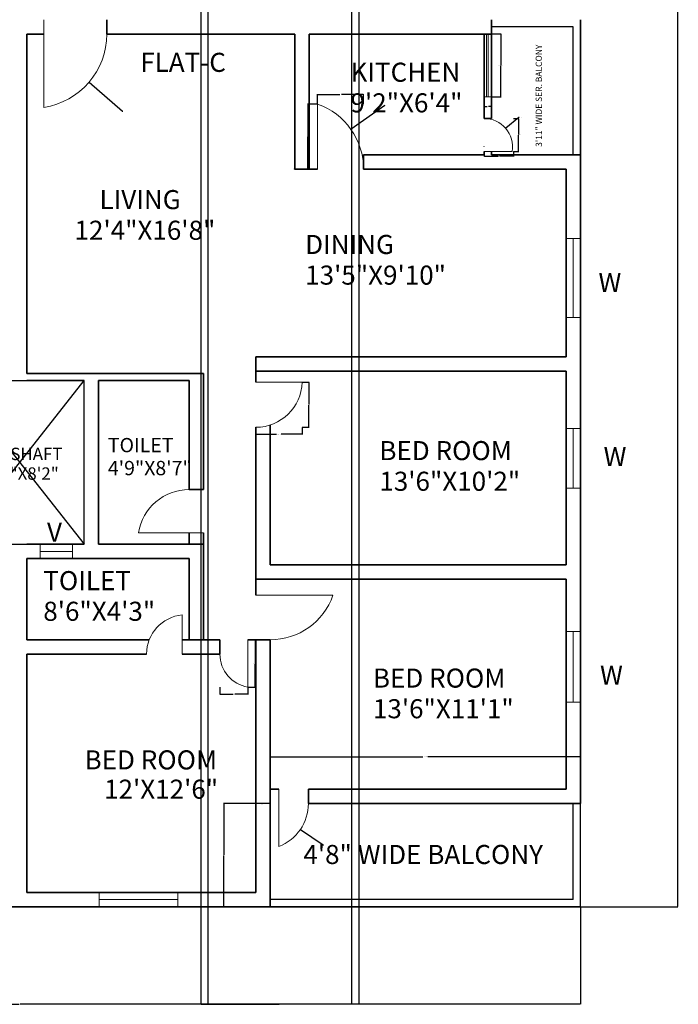
# Model space of a CAD drawing. Units: feet. Extents: x 5816 to 6644, y 25475 to 26788.
# Tile 2 of 23: x 6230 to 6644, y 25475 to 26094. Entities that reach past the tile are written whole.
import ezdxf

# ---------------------------------------------------------------- set-up
doc = ezdxf.new("R2010")
doc.units = ezdxf.units.FT
for name, color, linetype, lineweight in [('A-ANNO-DIMS', 2, 'Continuous', 13), ('A-ANNO-TEXT', 7, 'Continuous', 18), ('A-AREA-IDEN', 7, 'Continuous', 18), ('A-DOOR', 3, 'Continuous', 18), ('A-FLOR-RAIL', 8, 'Continuous', 25), ('A-FLOR-SHFT', 8, 'Continuous', 25), ('A-GLAZ', 4, 'Continuous', 18), ('A-WALL', 7, 'Continuous', 35)]:
    doc.layers.add(name, color=color, linetype=linetype, lineweight=lineweight)
doc.styles.get("Standard").update_dxf_attribs({"font": 'arial.ttf'})
doc.dimstyles.get("Standard").update_dxf_attribs({"dimtxt": 0.18, "dimasz": 0.18, "dimexe": 0.18, "dimexo": 0.0625, "dimgap": 0.09, "dimtad": 0, "dimtih": 1, "dimtoh": 1, "dimdec": 4, "dimzin": 0, "dimdsep": 46, "dimtxsty": 'Standard', "dimcen": 0.09, "dimadec": 0, "dimazin": 0, "dimtfac": 1, "dimtdec": 4, "dimtofl": 0, "dimtmove": 0, "dimatfit": 3, "dimfxl": 1, "dimtolj": 1, "dimtzin": 0, "dimarcsym": 0})

# ---------------------------------------------------------------- blocks, each defined once
blk = doc.blocks.new('DOOR-BALCONY')
blk.add_line((0, 36.11), (0, 0))
blk.add_arc((10.54, 9), 29.09, 111.24329, 180)
blk = doc.blocks.new('DOOR-BEDROOM-INNER')
blk.add_line((0, 29.82), (0, 0))
blk.add_arc((-3.45, 9), 21.11, 0, 80.59123)
blk = doc.blocks.new('DOOR-BEDROOM-BALCONY')
blk.add_line((-48.41, 0), (0, 0))
blk.add_arc((-9, -13.73), 41.74, 90, 160.78776)
blk = doc.blocks.new('DOOR-BEDROOM-SIDE')
blk.add_line((-28.98, 0), (0, 0))
blk.add_arc((0.03, -0.75), 29.02, 90, 178.52212)
blk = doc.blocks.new('DOOR-KITCHEN')
blk.add_line((0, -40.87), (0, 0))
blk.add_arc((14.45, 0), 43.35, 180, 250.52864)
blk = doc.blocks.new('DOOR-SERVICE-BALCONY')
blk.add_line((-17.56, 0), (0, 0))
blk.add_arc((0, -2.91), 17.8, 170.58679, 270)
blk = doc.blocks.new('DOOR-FLAT-ENTRY')
blk.add_line((0, 55.13), (0, 0))
blk.add_arc((7.05, 9.01), 46.66, 98.693, 180)
blk = doc.blocks.new('DOOR-BATH-ENSUITE')
blk.add_line((0, -24.59), (0, 0))
blk.add_arc((-2.33, 0.02), 24.72, 275.40734, 0)
blk = doc.blocks.new('DOOR-BATH-HALL')
blk.add_line((40.72, 0), (0, 0))
blk.add_arc((9, 4.86), 32.09, 270, 351.28818)
blk = doc.blocks.new('WIN-DINING')
for p, q in [((0, 0), (9, 0)), ((4.5, 0), (4.5, -49.84)), ((0, -49.84), (9, -49.84))]:
    blk.add_line(p, q)
blk = doc.blocks.new('WIN-BEDROOM-SIDE')
for p, q in [((0, 0), (9, 0)), ((4.5, 0), (4.5, -37.54)), ((0, -37.54), (9, -37.54))]:
    blk.add_line(p, q)
blk = doc.blocks.new('WIN-BEDROOM-BALCONY')
for p, q in [((0, 0), (9, 0)), ((4.5, 0), (4.5, -44.28)), ((0, -44.28), (9, -44.28))]:
    blk.add_line(p, q)
blk = doc.blocks.new('WIN-BEDROOM-INNER')
for p, q in [((49.5, 0), (49.5, -9)), ((0, 0), (0, -9)), ((0, -4.5), (49.5, -4.5))]:
    blk.add_line(p, q)
blk = doc.blocks.new('WIN-KITCHEN')
for p, q in [((0, 0), (4.5, 0)), ((2, 0), (2, -39.61)), ((3, 0), (3, -39.61))]:
    blk.add_line(p, q)
blk = doc.blocks.new('WIN-VENT-NARROW')
for p, q in [((0, 0), (0, -9)), ((20.24, 0), (20.24, -9)), ((0, -4.5), (20.24, -4.5))]:
    blk.add_line(p, q)
blk = doc.blocks.new('VENT-SHAFT')
for p, q in [((0, 0), (0, 103)), ((0, 103), (81, 103)), ((0, 103), (81, 0)), ((0, 0), (81, 103)), ((81, 103), (45, 103)), ((81, 0), (81, 103)), ((0, 0), (81, 0)), ((81, 0), (45, 0))]:
    blk.add_line(p, q)
blk = doc.blocks.new('RAIL-BALCONY-CORNER')
for p, q in [((0, 0), (0, -65)), ((0, 0), (195, 0)), ((4.5, -4.5), (4.5, -65)), ((4.5, -4.5), (195, -4.5))]:
    blk.add_line(p, q)
blk = doc.blocks.new('*D21')
at = {"layer": 'A-ANNO-DIMS', "color": 0, "lineweight": -2, "transparency": 16777216}
for p, q in [((6373.37, 25704.34), (6377.96, 25704.34)), ((6377.78, 25704.16), (6377.78, 25689.61)), ((6377.78, 25674.69), (6377.78, 25689.24)), ((6373.37, 25674.51), (6377.96, 25674.51))]:
    blk.add_line(p, q, dxfattribs=at)
at = {"layer": 'A-ANNO-DIMS', "color": 0, "transparency": 16777216}
for points in [[(6377.75, 25704.16), (6377.81, 25704.16), (6377.78, 25704.34)], [(6377.75, 25674.69), (6377.81, 25674.69), (6377.78, 25674.51)]]:
    blk.add_solid(points, dxfattribs=at)
at = {"layer": 'Defpoints', "color": 0, "transparency": 16777216}
for p in [(6373.31, 25704.34), (6373.31, 25674.51), (6377.78, 25674.51)]:
    blk.add_point(p, dxfattribs=at)
at = {"layer": 'A-ANNO-DIMS', "color": 0, "transparency": 16777216, "insert": (6377.78, 25689.42), "char_height": 0.18, "attachment_point": 5}
blk.add_mtext('\\A1;INNER BR DOOR 30 TYP.', dxfattribs=at)
blk = doc.blocks.new('*D22')
at = {"layer": 'A-ANNO-DIMS', "color": 0, "lineweight": -2, "transparency": 16777216}
for p, q in [((6355.65, 25674.45), (6355.65, 25669.86)), ((6373.31, 25674.45), (6373.31, 25669.86)), ((6355.83, 25670.04), (6363.96, 25670.04)), ((6373.13, 25670.04), (6365, 25670.04))]:
    blk.add_line(p, q, dxfattribs=at)
at = {"layer": 'A-ANNO-DIMS', "color": 0, "transparency": 16777216}
for points in [[(6355.83, 25670.07), (6355.83, 25670.01), (6355.65, 25670.04)], [(6373.13, 25670.07), (6373.13, 25670.01), (6373.31, 25670.04)]]:
    blk.add_solid(points, dxfattribs=at)
at = {"layer": 'Defpoints', "color": 0, "transparency": 16777216}
for p in [(6355.65, 25674.51), (6373.31, 25674.51), (6355.65, 25670.04)]:
    blk.add_point(p, dxfattribs=at)
at = {"layer": 'A-ANNO-DIMS', "color": 0, "transparency": 16777216, "insert": (6364.48, 25670.04), "char_height": 0.18, "attachment_point": 5}
blk.add_mtext('\\A1;18 TYP.', dxfattribs=at)
blk = doc.blocks.new('*D25')
at = {"layer": 'A-ANNO-DIMS', "color": 0, "lineweight": -2, "transparency": 16777216}
for p, q in [((6378.28, 25837.91), (6378.28, 25833.45)), ((6378.46, 25833.63), (6391.31, 25833.63)), ((6407.11, 25833.63), (6394.26, 25833.63)), ((6407.29, 25837.91), (6407.29, 25833.45))]:
    blk.add_line(p, q, dxfattribs=at)
at = {"layer": 'A-ANNO-DIMS', "color": 0, "transparency": 16777216}
for points in [[(6378.46, 25833.66), (6378.46, 25833.6), (6378.28, 25833.63)], [(6407.11, 25833.66), (6407.11, 25833.6), (6407.29, 25833.63)]]:
    blk.add_solid(points, dxfattribs=at)
at = {"layer": 'Defpoints', "color": 0, "transparency": 16777216}
for p in [(6378.28, 25837.98), (6378.28, 25833.63), (6407.29, 25837.98)]:
    blk.add_point(p, dxfattribs=at)
at = {"layer": 'A-ANNO-DIMS', "color": 0, "transparency": 16777216, "insert": (6392.78, 25833.63), "char_height": 0.18, "attachment_point": 5}
blk.add_mtext('\\A1;SIDE BR DOOR 29 TYP.', dxfattribs=at)
blk = doc.blocks.new('*D26')
at = {"layer": 'A-ANNO-DIMS', "color": 0, "lineweight": -2, "transparency": 16777216}
for p, q in [((6407.35, 25866.24), (6411.82, 25866.24)), ((6411.64, 25866.06), (6411.64, 25852.29)), ((6411.64, 25838.16), (6411.64, 25851.93)), ((6407.35, 25837.98), (6411.82, 25837.98))]:
    blk.add_line(p, q, dxfattribs=at)
at = {"layer": 'A-ANNO-DIMS', "color": 0, "transparency": 16777216}
for points in [[(6411.61, 25866.06), (6411.67, 25866.06), (6411.64, 25866.24)], [(6411.61, 25838.16), (6411.67, 25838.16), (6411.64, 25837.98)]]:
    blk.add_solid(points, dxfattribs=at)
at = {"layer": 'Defpoints', "color": 0, "transparency": 16777216}
for p in [(6407.29, 25866.24), (6407.29, 25837.98), (6411.64, 25837.98)]:
    blk.add_point(p, dxfattribs=at)
at = {"layer": 'A-ANNO-DIMS', "color": 0, "transparency": 16777216, "insert": (6411.64, 25852.11), "char_height": 0.18, "attachment_point": 5}
blk.add_mtext('\\A1;28 TYP.', dxfattribs=at)
blk = doc.blocks.new('*D27')
at = {"layer": 'A-ANNO-DIMS', "color": 0, "lineweight": -2, "transparency": 16777216}
for p, q in [((6417.03, 26041.21), (6410.78, 26041.21)), ((6410.96, 26041.03), (6410.96, 26020.95)), ((6410.96, 26000.52), (6410.96, 26020.59)), ((6417.03, 26000.34), (6410.78, 26000.34))]:
    blk.add_line(p, q, dxfattribs=at)
at = {"layer": 'A-ANNO-DIMS', "color": 0, "transparency": 16777216}
for points in [[(6410.93, 26041.03), (6410.99, 26041.03), (6410.96, 26041.21)], [(6410.93, 26000.52), (6410.99, 26000.52), (6410.96, 26000.34)]]:
    blk.add_solid(points, dxfattribs=at)
at = {"layer": 'Defpoints', "color": 0, "transparency": 16777216}
for p in [(6417.09, 26041.21), (6410.96, 26000.34), (6417.09, 26000.34)]:
    blk.add_point(p, dxfattribs=at)
at = {"layer": 'A-ANNO-DIMS', "color": 0, "transparency": 16777216, "insert": (6410.96, 26020.77), "char_height": 0.18, "attachment_point": 5}
blk.add_mtext('\\A1;KITCHEN DOOR 41 TYP.', dxfattribs=at)
blk = doc.blocks.new('*D28')
at = {"layer": 'A-ANNO-DIMS', "color": 0, "lineweight": -2, "transparency": 16777216}
for p, q in [((6417.09, 26041.27), (6417.09, 26047.52)), ((6417.27, 26047.34), (6431.01, 26047.34)), ((6445.81, 26047.34), (6432.07, 26047.34)), ((6445.99, 26041.27), (6445.99, 26047.52))]:
    blk.add_line(p, q, dxfattribs=at)
at = {"layer": 'A-ANNO-DIMS', "color": 0, "transparency": 16777216}
for points in [[(6417.27, 26047.37), (6417.27, 26047.31), (6417.09, 26047.34)], [(6445.81, 26047.37), (6445.81, 26047.31), (6445.99, 26047.34)]]:
    blk.add_solid(points, dxfattribs=at)
at = {"layer": 'Defpoints', "color": 0, "transparency": 16777216}
for p in [(6417.09, 26047.34), (6417.09, 26041.21), (6445.99, 26041.21)]:
    blk.add_point(p, dxfattribs=at)
at = {"layer": 'A-ANNO-DIMS', "color": 0, "transparency": 16777216, "insert": (6431.54, 26047.34), "char_height": 0.18, "attachment_point": 5}
blk.add_mtext('\\A1;29 TYP.', dxfattribs=at)
blk = doc.blocks.new('*D29')
at = {"layer": 'A-ANNO-DIMS', "color": 0, "lineweight": -2, "transparency": 16777216}
for p, q in [((6540.29, 26032.22), (6543.51, 26032.22)), ((6543.33, 26032.04), (6543.33, 26022.05)), ((6543.33, 26011.7), (6543.33, 26021.69)), ((6540.29, 26011.52), (6543.51, 26011.52))]:
    blk.add_line(p, q, dxfattribs=at)
at = {"layer": 'A-ANNO-DIMS', "color": 0, "transparency": 16777216}
for points in [[(6543.3, 26032.04), (6543.36, 26032.04), (6543.33, 26032.22)], [(6543.3, 26011.7), (6543.36, 26011.7), (6543.33, 26011.52)]]:
    blk.add_solid(points, dxfattribs=at)
at = {"layer": 'Defpoints', "color": 0, "transparency": 16777216}
for p in [(6540.23, 26032.22), (6540.23, 26011.52), (6543.33, 26011.52)]:
    blk.add_point(p, dxfattribs=at)
at = {"layer": 'A-ANNO-DIMS', "color": 0, "transparency": 16777216, "insert": (6543.33, 26021.87), "char_height": 0.18, "attachment_point": 5}
blk.add_mtext('\\A1;SERVICE DOOR 21 TYP.', dxfattribs=at)
blk = doc.blocks.new('*D30')
at = {"layer": 'A-ANNO-DIMS', "color": 0, "lineweight": -2, "transparency": 16777216}
for p, q in [((6521.81, 26011.45), (6521.81, 26008.23)), ((6521.99, 26008.41), (6530.5, 26008.41)), ((6540.05, 26008.41), (6531.54, 26008.41)), ((6540.23, 26011.45), (6540.23, 26008.23))]:
    blk.add_line(p, q, dxfattribs=at)
at = {"layer": 'A-ANNO-DIMS', "color": 0, "transparency": 16777216}
for points in [[(6521.99, 26008.44), (6521.99, 26008.38), (6521.81, 26008.41)], [(6540.05, 26008.44), (6540.05, 26008.38), (6540.23, 26008.41)]]:
    blk.add_solid(points, dxfattribs=at)
at = {"layer": 'Defpoints', "color": 0, "transparency": 16777216}
for p in [(6521.81, 26011.52), (6521.81, 26008.41), (6540.23, 26011.52)]:
    blk.add_point(p, dxfattribs=at)
at = {"layer": 'A-ANNO-DIMS', "color": 0, "transparency": 16777216, "insert": (6531.02, 26008.41), "char_height": 0.18, "attachment_point": 5}
blk.add_mtext('\\A1;18 TYP.', dxfattribs=at)
blk = doc.blocks.new('*D45')
at = {"layer": 'A-ANNO-DIMS', "color": 0, "lineweight": -2, "transparency": 16777216}
for p, q in [((6526.37, 26085.34), (6532.43, 26085.34)), ((6532.25, 26085.16), (6532.25, 26065.72)), ((6532.25, 26045.91), (6532.25, 26065.35)), ((6526.37, 26045.73), (6532.43, 26045.73))]:
    blk.add_line(p, q, dxfattribs=at)
at = {"layer": 'A-ANNO-DIMS', "color": 0, "transparency": 16777216}
for points in [[(6532.22, 26085.16), (6532.28, 26085.16), (6532.25, 26085.34)], [(6532.22, 26045.91), (6532.28, 26045.91), (6532.25, 26045.73)]]:
    blk.add_solid(points, dxfattribs=at)
at = {"layer": 'Defpoints', "color": 0, "transparency": 16777216}
for p in [(6526.31, 26085.34), (6526.31, 26045.73), (6532.25, 26045.73)]:
    blk.add_point(p, dxfattribs=at)
at = {"layer": 'A-ANNO-DIMS', "color": 0, "transparency": 16777216, "insert": (6532.25, 26065.53), "char_height": 0.18, "attachment_point": 5}
blk.add_mtext('\\A1;KITCHEN WINDOW 40 TYP.', dxfattribs=at)
blk = doc.blocks.new('*D46')
at = {"layer": 'A-ANNO-DIMS', "color": 0, "lineweight": -2, "transparency": 16777216}
for p, q in [((6521.81, 26045.67), (6521.81, 26039.61)), ((6526.31, 26045.67), (6526.31, 26039.61)), ((6521.99, 26039.79), (6523.6, 26039.79)), ((6526.13, 26039.79), (6524.52, 26039.79))]:
    blk.add_line(p, q, dxfattribs=at)
at = {"layer": 'A-ANNO-DIMS', "color": 0, "transparency": 16777216}
for points in [[(6521.99, 26039.82), (6521.99, 26039.76), (6521.81, 26039.79)], [(6526.13, 26039.82), (6526.13, 26039.76), (6526.31, 26039.79)]]:
    blk.add_solid(points, dxfattribs=at)
at = {"layer": 'Defpoints', "color": 0, "transparency": 16777216}
for p in [(6521.81, 26045.73), (6526.31, 26045.73), (6521.81, 26039.79)]:
    blk.add_point(p, dxfattribs=at)
at = {"layer": 'A-ANNO-DIMS', "color": 0, "transparency": 16777216, "insert": (6524.06, 26039.79), "char_height": 0.18, "attachment_point": 5}
blk.add_mtext('\\A1;5 TYP.', dxfattribs=at)
blk = doc.blocks.new('*D47')
at = {"layer": 'A-ANNO-DIMS', "color": 0, "lineweight": -2, "transparency": 16777216}
for p, q in [((6387.31, 25601.4), (6387.31, 25630.77)), ((6387.49, 25630.59), (6483.27, 25630.59)), ((6582.13, 25630.59), (6486.36, 25630.59)), ((6582.31, 25601.4), (6582.31, 25630.77))]:
    blk.add_line(p, q, dxfattribs=at)
at = {"layer": 'A-ANNO-DIMS', "color": 0, "transparency": 16777216}
for points in [[(6387.49, 25630.62), (6387.49, 25630.56), (6387.31, 25630.59)], [(6582.13, 25630.62), (6582.13, 25630.56), (6582.31, 25630.59)]]:
    blk.add_solid(points, dxfattribs=at)
at = {"layer": 'Defpoints', "color": 0, "transparency": 16777216}
for p in [(6387.31, 25630.59), (6387.31, 25601.34), (6582.31, 25601.34)]:
    blk.add_point(p, dxfattribs=at)
at = {"layer": 'A-ANNO-DIMS', "color": 0, "transparency": 16777216, "insert": (6484.81, 25630.59), "char_height": 0.18, "attachment_point": 5}
blk.add_mtext('\\A1;BALCONY RAIL 195 TYP.', dxfattribs=at)
blk = doc.blocks.new('*D48')
at = {"layer": 'A-ANNO-DIMS', "color": 0, "lineweight": -2, "transparency": 16777216}
for p, q in [((6387.25, 25601.34), (6357.88, 25601.34)), ((6358.06, 25601.16), (6358.06, 25569.02)), ((6358.06, 25536.52), (6358.06, 25568.65)), ((6387.25, 25536.34), (6357.88, 25536.34))]:
    blk.add_line(p, q, dxfattribs=at)
at = {"layer": 'A-ANNO-DIMS', "color": 0, "transparency": 16777216}
for points in [[(6358.03, 25601.16), (6358.09, 25601.16), (6358.06, 25601.34)], [(6358.03, 25536.52), (6358.09, 25536.52), (6358.06, 25536.34)]]:
    blk.add_solid(points, dxfattribs=at)
at = {"layer": 'Defpoints', "color": 0, "transparency": 16777216}
for p in [(6387.31, 25601.34), (6358.06, 25536.34), (6387.31, 25536.34)]:
    blk.add_point(p, dxfattribs=at)
at = {"layer": 'A-ANNO-DIMS', "color": 0, "transparency": 16777216, "insert": (6358.06, 25568.84), "char_height": 0.18, "attachment_point": 5}
blk.add_mtext('\\A1;65 TYP.', dxfattribs=at)
blk = doc.blocks.new('*D55')
at = {"layer": 'A-ANNO-DIMS', "color": 0, "lineweight": -2, "transparency": 16777216}
for p, q in [((5877.31, 25536.27), (5877.31, 25475.01)), ((6582.31, 25536.27), (6582.31, 25475.01)), ((5877.49, 25475.19), (6229.52, 25475.19)), ((6582.13, 25475.19), (6230.1, 25475.19))]:
    blk.add_line(p, q, dxfattribs=at)
at = {"layer": 'A-ANNO-DIMS', "color": 0, "transparency": 16777216}
for points in [[(5877.49, 25475.22), (5877.49, 25475.16), (5877.31, 25475.19)], [(6582.13, 25475.22), (6582.13, 25475.16), (6582.31, 25475.19)]]:
    blk.add_solid(points, dxfattribs=at)
at = {"layer": 'Defpoints', "color": 0, "transparency": 16777216}
for p in [(5877.31, 25536.34), (6582.31, 25536.34), (6582.31, 25475.19)]:
    blk.add_point(p, dxfattribs=at)
at = {"layer": 'A-ANNO-DIMS', "color": 0, "transparency": 16777216, "insert": (6229.81, 25475.19), "char_height": 0.18, "attachment_point": 5}
blk.add_mtext('\\A1;705', dxfattribs=at)
blk = doc.blocks.new('*D56')
at = {"layer": 'A-ANNO-DIMS', "color": 0, "lineweight": -2, "transparency": 16777216}
for p, q in [((6582.37, 26726.58), (6643.64, 26726.58)), ((6643.46, 26726.4), (6643.46, 26131.64)), ((6643.46, 25536.52), (6643.46, 26131.28)), ((6582.37, 25536.34), (6643.64, 25536.34))]:
    blk.add_line(p, q, dxfattribs=at)
at = {"layer": 'A-ANNO-DIMS', "color": 0, "transparency": 16777216}
for points in [[(6643.43, 26726.4), (6643.49, 26726.4), (6643.46, 26726.58)], [(6643.43, 25536.52), (6643.49, 25536.52), (6643.46, 25536.34)]]:
    blk.add_solid(points, dxfattribs=at)
at = {"layer": 'Defpoints', "color": 0, "transparency": 16777216}
for p in [(6582.31, 26726.58), (6643.46, 26726.58), (6582.31, 25536.34)]:
    blk.add_point(p, dxfattribs=at)
at = {"layer": 'A-ANNO-DIMS', "color": 0, "transparency": 16777216, "insert": (6643.46, 26131.46), "char_height": 0.18, "attachment_point": 5}
blk.add_mtext('\\A1;1190.2', dxfattribs=at)
blk = doc.blocks.new('*D59')
at = {"layer": 'A-ANNO-DIMS', "color": 0, "lineweight": -2, "transparency": 16777216}
for p, q in [((6343.68, 26168.52), (6343.68, 25475.01)), ((6442.98, 26168.59), (6442.98, 25475.01)), ((6343.86, 25475.19), (6393, 25475.19)), ((6442.8, 25475.19), (6393.65, 25475.19))]:
    blk.add_line(p, q, dxfattribs=at)
at = {"layer": 'A-ANNO-DIMS', "color": 0, "transparency": 16777216}
for points in [[(6343.86, 25475.22), (6343.86, 25475.16), (6343.68, 25475.19)], [(6442.8, 25475.22), (6442.8, 25475.16), (6442.98, 25475.19)]]:
    blk.add_solid(points, dxfattribs=at)
at = {"layer": 'Defpoints', "color": 0, "transparency": 16777216}
for p in [(6343.68, 26168.58), (6442.98, 26168.65), (6442.98, 25475.19)]:
    blk.add_point(p, dxfattribs=at)
at = {"layer": 'A-ANNO-DIMS', "color": 0, "transparency": 16777216, "insert": (6393.33, 25475.19), "char_height": 0.18, "attachment_point": 5}
blk.add_mtext('\\A1;99.3', dxfattribs=at)
blk = doc.blocks.new('*D73')
at = {"layer": 'A-ANNO-DIMS', "color": 0, "lineweight": -2, "transparency": 16777216}
for p, q in [((6348.18, 26111.07), (6348.18, 25475.01)), ((6438.48, 26111.07), (6438.48, 25475.01)), ((6348.36, 25475.19), (6393, 25475.19)), ((6438.3, 25475.19), (6393.65, 25475.19))]:
    blk.add_line(p, q, dxfattribs=at)
at = {"layer": 'A-ANNO-DIMS', "color": 0, "transparency": 16777216}
for points in [[(6348.36, 25475.22), (6348.36, 25475.16), (6348.18, 25475.19)], [(6438.3, 25475.22), (6438.3, 25475.16), (6438.48, 25475.19)]]:
    blk.add_solid(points, dxfattribs=at)
at = {"layer": 'Defpoints', "color": 0, "transparency": 16777216}
for p in [(6348.18, 26111.13), (6438.48, 26111.13), (6438.48, 25475.19)]:
    blk.add_point(p, dxfattribs=at)
at = {"layer": 'A-ANNO-DIMS', "color": 0, "transparency": 16777216, "insert": (6393.33, 25475.19), "char_height": 0.18, "attachment_point": 5}
blk.add_mtext('\\A1;90.3', dxfattribs=at)
blk = doc.blocks.new('*D74')
at = {"layer": 'A-ANNO-DIMS', "color": 0, "lineweight": -2, "transparency": 16777216}
for p, q in [((6237.79, 26085.33), (6237.97, 26085.33)), ((6237.88, 26085.24), (6237.88, 26085.42)), ((6294.52, 26036.69), (6273.42, 26054.81)), ((6294.7, 26036.69), (6294.52, 26036.69))]:
    blk.add_line(p, q, dxfattribs=at)
at = {"layer": 'A-ANNO-DIMS', "color": 0, "transparency": 16777216}
blk.add_solid([(6273.44, 26054.84), (6273.4, 26054.79), (6273.28, 26054.93)], dxfattribs=at)
at = {"layer": 'Defpoints', "color": 0, "transparency": 16777216}
for p in [(6237.88, 26085.33), (6273.28, 26054.93)]:
    blk.add_point(p, dxfattribs=at)
at = {"layer": 'A-ANNO-DIMS', "color": 0, "transparency": 16777216, "insert": (6295.38, 26036.69), "char_height": 0.18, "attachment_point": 5}
blk.add_mtext('\\A1;4X R46.66', dxfattribs=at)
blk = doc.blocks.new('*D75')
at = {"layer": 'A-ANNO-DIMS', "color": 0, "lineweight": -2, "transparency": 16777216}
for p, q in [((6459.27, 26040.38), (6438.18, 26025.47)), ((6459.45, 26040.38), (6459.27, 26040.38)), ((6402.55, 26000.34), (6402.73, 26000.34)), ((6402.64, 26000.25), (6402.64, 26000.43))]:
    blk.add_line(p, q, dxfattribs=at)
at = {"layer": 'A-ANNO-DIMS', "color": 0, "transparency": 16777216}
blk.add_solid([(6438.17, 26025.49), (6438.2, 26025.44), (6438.04, 26025.36)], dxfattribs=at)
at = {"layer": 'Defpoints', "color": 0, "transparency": 16777216}
for p in [(6438.04, 26025.36), (6402.64, 26000.34)]:
    blk.add_point(p, dxfattribs=at)
at = {"layer": 'A-ANNO-DIMS', "color": 0, "transparency": 16777216, "insert": (6460.13, 26040.38), "char_height": 0.18, "attachment_point": 5}
blk.add_mtext('\\A1;4X R43.35', dxfattribs=at)
blk = doc.blocks.new('*D78')
at = {"layer": 'A-ANNO-DIMS', "color": 0, "lineweight": -2, "transparency": 16777216}
for p, q in [((6382.13, 25601.34), (6382.31, 25601.34)), ((6382.22, 25601.25), (6382.22, 25601.43)), ((6420.64, 25575.06), (6406.38, 25584.81)), ((6420.82, 25575.06), (6420.64, 25575.06))]:
    blk.add_line(p, q, dxfattribs=at)
at = {"layer": 'A-ANNO-DIMS', "color": 0, "transparency": 16777216}
blk.add_solid([(6406.4, 25584.83), (6406.36, 25584.78), (6406.23, 25584.91)], dxfattribs=at)
at = {"layer": 'Defpoints', "color": 0, "transparency": 16777216}
for p in [(6382.22, 25601.34), (6406.23, 25584.91)]:
    blk.add_point(p, dxfattribs=at)
at = {"layer": 'A-ANNO-DIMS', "color": 0, "transparency": 16777216, "insert": (6421.49, 25575.06), "char_height": 0.18, "attachment_point": 5}
blk.add_mtext('\\A1;4X R29.09', dxfattribs=at)
blk = doc.blocks.new('*D82')
at = {"layer": 'A-ANNO-DIMS', "color": 0, "lineweight": -2, "transparency": 16777216}
for p, q in [((6543.53, 26032.84), (6535.52, 26026.05)), ((6543.71, 26032.84), (6543.53, 26032.84)), ((6521.72, 26014.43), (6521.9, 26014.43)), ((6521.81, 26014.34), (6521.81, 26014.52))]:
    blk.add_line(p, q, dxfattribs=at)
at = {"layer": 'A-ANNO-DIMS', "color": 0, "transparency": 16777216}
blk.add_solid([(6535.5, 26026.08), (6535.54, 26026.03), (6535.39, 26025.94)], dxfattribs=at)
at = {"layer": 'Defpoints', "color": 0, "transparency": 16777216}
for p in [(6535.39, 26025.94), (6521.81, 26014.43)]:
    blk.add_point(p, dxfattribs=at)
at = {"layer": 'A-ANNO-DIMS', "color": 0, "transparency": 16777216, "insert": (6544.46, 26032.84), "char_height": 0.18, "attachment_point": 5}
blk.add_mtext('\\A1;4X R17.798', dxfattribs=at)

msp = doc.modelspace()

# ---------------------------------------------------------------- linework, layer by layer
at = {"layer": 'A-FLOR-RAIL'}
msp.add_lwpolyline([(6577.8119, 26009.3368), (6577.8119, 26089.8368), (6526.3119, 26089.8368)], dxfattribs=at)
at = {"layer": 'A-WALL'}
for p, q in [((6284.5408, 26085.3298), (6284.5408, 26094.3368)), ((6526.3119, 26032.2246), (6526.3119, 26094.3368)), ((6582.3119, 26000.3368), (6582.3119, 26094.3368)), ((6244.9332, 26085.3368), (6234.3119, 26085.3368)), ((6234.3119, 25871.8368), (6234.3119, 26085.3368)), ((6402.8119, 26085.3368), (6284.5408, 26085.3368)), ((6402.8119, 26085.3368), (6402.8119, 26009.3368)), ((6526.3119, 26085.3368), (6411.8119, 26085.3368)), ((6411.8119, 26085.3368), (6411.8119, 26000.3368)), ((6521.8119, 26032.2246), (6521.8119, 26085.3368)), ((6526.3119, 26032.2246), (6521.8119, 26032.2246)), ((6402.8119, 26009.3368), (6402.8119, 26000.3368)), ((6521.8119, 26009.3368), (6445.9911, 26009.3368)), ((6445.9911, 26000.3368), (6445.9911, 26009.3368)), ((6521.8119, 26009.3368), (6521.8119, 26011.5155)), ((6526.3119, 26009.3368), (6526.3119, 26011.5155)), ((6573.3119, 26009.3368), (6526.3119, 26009.3368)), ((6573.3119, 26009.3368), (6582.3119, 26009.3368)), ((6582.3119, 25610.3368), (6582.3119, 26009.3368)), ((6582.3119, 25751.3368), (6582.3119, 26009.3368)), ((6417.0917, 26000.3368), (6402.8119, 26000.3368)), ((6573.3119, 26000.3368), (6445.9911, 26000.3368)), ((6573.3119, 25882.3368), (6573.3119, 26000.3368)), ((6582.3119, 25882.3368), (6582.3119, 26000.3368)), ((6573.3119, 25882.3368), (6378.3119, 25882.3368)), ((6378.3119, 25866.2444), (6378.3119, 25882.3368)), ((6336.3119, 25871.8368), (6234.3119, 25871.8368)), ((6336.3119, 25871.8368), (6345.3119, 25871.8368)), ((6345.3119, 25798.8236), (6345.3119, 25871.8368)), ((6573.3119, 25873.3368), (6378.3119, 25873.3368)), ((6573.3119, 25751.3368), (6573.3119, 25873.3368)), ((6336.3119, 25867.3368), (6279.3119, 25867.3368)), ((6279.3119, 25867.3368), (6279.3119, 25764.3368)), ((6336.3119, 25798.8236), (6336.3119, 25867.3368)), ((6387.3119, 25751.3368), (6387.3119, 25839.4181)), ((6378.3119, 25732.3387), (6378.3119, 25837.9771)), ((6336.3119, 25798.8236), (6345.3119, 25798.8236)), ((6336.3119, 25764.3368), (6336.3119, 25771.5927)), ((6345.3119, 25704.3368), (6345.3119, 25771.5927)), ((6345.3119, 25764.3368), (6279.3119, 25764.3368)), ((6336.3119, 25755.3368), (6234.3119, 25755.3368)), ((6234.3119, 25755.3368), (6234.3119, 25704.3368)), ((6336.3119, 25704.3368), (6336.3119, 25755.3368)), ((6573.3119, 25751.3368), (6387.3119, 25751.3368)), ((6573.3119, 25742.3368), (6378.3119, 25742.3368)), ((6378.3119, 25742.3368), (6378.3119, 25732.3387)), ((6573.3119, 25610.3368), (6573.3119, 25742.3368)), ((6234.3119, 25704.3368), (6311.248, 25704.3368)), ((6234.3119, 25704.3368), (6311.248, 25704.3368)), ((6331.936, 25704.3368), (6355.6538, 25704.3368)), ((6331.936, 25704.3368), (6336.3119, 25704.3368)), ((6355.6538, 25695.3368), (6355.6538, 25704.3368)), ((6373.3112, 25704.3368), (6387.3119, 25704.3368)), ((6378.3119, 25704.3368), (6378.3119, 25594.1569)), ((6387.3119, 25704.3368), (6387.3119, 25594.1569)), ((6234.3119, 25545.3368), (6234.3119, 25695.3368)), ((6234.3119, 25695.3368), (6309.5426, 25695.3368)), ((6331.936, 25695.3368), (6355.6538, 25695.3368)), ((6392.7622, 25610.3368), (6387.3119, 25610.3368)), ((6573.3119, 25610.3368), (6411.3119, 25610.3368)), ((6411.3119, 25610.3368), (6411.3119, 25601.3368)), ((6582.3119, 25601.3368), (6582.3119, 25610.3368)), ((6378.3119, 25601.3368), (6378.3119, 25545.3368)), ((6387.3119, 25601.3368), (6387.3119, 25536.3368)), ((6582.3119, 25601.3368), (6411.3119, 25601.3368)), ((6378.3119, 25545.3368), (6234.3119, 25545.3368)), ((5877.3119, 25536.3368), (6279.7398, 25536.3368)), ((6582.3119, 25536.3368), (6234.3119, 25536.3368))]:
    msp.add_line(p, q, dxfattribs=at)

# ---------------------------------------------------------------- block references
at = {"layer": 'A-DOOR', "rotation": 180}
for name, p in [('DOOR-FLAT-ENTRY', (6244.9332, 26094.3368)), ('DOOR-KITCHEN', (6417.0917, 26000.3368)), ('DOOR-SERVICE-BALCONY', (6521.8119, 26011.5155)), ('DOOR-BEDROOM-SIDE', (6378.3119, 25866.2444)), ('DOOR-BATH-HALL', (6345.3119, 25771.5927)), ('DOOR-BEDROOM-BALCONY', (6378.3119, 25732.3387)), ('DOOR-BATH-ENSUITE', (6331.936, 25695.3368)), ('DOOR-BEDROOM-INNER', (6373.3112, 25704.3368)), ('DOOR-BALCONY', (6392.7622, 25610.3368))]:
    msp.add_blockref(name, p, dxfattribs=at)
at = {"layer": 'A-FLOR-RAIL', "rotation": 180}
msp.add_blockref('RAIL-BALCONY-CORNER', (6582.3119, 25536.3368), dxfattribs=at)
at = {"layer": 'A-FLOR-SHFT'}
msp.add_blockref('VENT-SHAFT', (6189.3119, 25764.3368), dxfattribs=at)
at = {"layer": 'A-GLAZ', "rotation": 180}
for name, p in [('WIN-KITCHEN', (6526.3119, 26045.731)), ('WIN-DINING', (6582.3119, 25906.9414)), ('WIN-BEDROOM-BALCONY', (6582.3119, 25665.1277))]:
    msp.add_blockref(name, p, dxfattribs=at)
at = {"layer": 'A-GLAZ'}
for name, p in [('WIN-BEDROOM-SIDE', (6573.3119, 25837.1796)), ('WIN-VENT-NARROW', (6242.7596, 25764.3368)), ('WIN-BEDROOM-INNER', (6279.7398, 25545.3368))]:
    msp.add_blockref(name, p, dxfattribs=at)

# ---------------------------------------------------------------- texts
at = {"layer": 'A-ANNO-DIMS'}
for s, height, p in [('9\'2"X6\'4"', 12, (6437.7909, 26036.0213)), ('12\'4"X16\'8"', 12, (6264.2851, 25955.8889)), ('13\'5"X9\'10"', 12, (6409.2785, 25927.6758)), ('4\'9"X8\'7"', 8.98988, (6285.2405, 25807.8127)), ('6\'7"X8\'2"', 7.77416, (6208.7805, 25804.961)), ('13\'6"X10\'2"', 12, (6455.9147, 25798.0042)), ('8\'6"X4\'3"', 12, (6244.6415, 25716.2184)), ('13\'6"X11\'1"', 12, (6451.861, 25654.9247)), ('12\'X12\'6"', 12, (6282.8763, 25604.3235))]:
    msp.add_text(s, height=height, dxfattribs=at).set_placement(p)
at = {"layer": 'A-ANNO-TEXT'}
for s, p in [('W', (6593.636, 25923.074)), ('W', (6596.8674, 25813.5301)), ('V', (6246.9756, 25766.0074)), ('W', (6594.6249, 25676.0997))]:
    msp.add_text(s, height=12, dxfattribs=at).set_placement(p)
at = {"layer": 'A-AREA-IDEN'}
msp.add_text('3\'11" WIDE SER. BALCONY', height=3.901456, rotation=90, dxfattribs=at).set_placement((6558.0829, 26014.3721))
for s, height, p in [('FLAT-C', 12, (6305.6106, 26061.5111)), ('KITCHEN', 12, (6437.7909, 26055.2983)), ('LIVING', 12, (6279.9748, 25975.1658)), ('DINING', 12, (6409.2785, 25946.9527)), ('TOILET', 8.98988, (6285.2405, 25822.2542)), ('BED ROOM', 12, (6455.9147, 25817.2811)), ('VENT SHAFT', 7.77416, (6195.225, 25817.342)), ('TOILET', 12, (6244.6415, 25735.4953)), ('BED ROOM', 12, (6451.861, 25674.2016)), ('BED ROOM', 12, (6270.5851, 25622.7534)), ('4\'8" WIDE BALCONY', 12, (6408.1538, 25563.2479))]:
    msp.add_text(s, height=height, dxfattribs=at).set_placement(p)

# ---------------------------------------------------------------- dimensions: what is measured, and where the dimension line sits
at = {"layer": 'A-ANNO-DIMS'}
dim = msp.add_linear_dim(base=(6643.4619, 26726.5846), p1=(6582.3119, 25536.3368), p2=(6582.3119, 26726.5846), angle=90, dimstyle='Standard', override={"dimdec": 1, "dimlfac": 1, "dimrnd": 0, "dimzin": 0, "dimdsep": 46, "dimlunit": 2}, dxfattribs=at)
dim.commit()
dim.dimension.update_dxf_attribs({"geometry": '*D56', "text_midpoint": (6643.4619, 26131.4607)})
for base, p1, p2, override, picture, middle in [((6442.9781, 25475.1868), (6343.6763, 26168.5846), (6442.9781, 26168.6509), {"dimdec": 1, "dimlfac": 1, "dimrnd": 0, "dimzin": 0, "dimdsep": 46, "dimlunit": 2}, '*D59', (6393.3272, 25475.1868)), ((6438.4781, 25475.1868), (6348.1763, 26111.129), (6438.4781, 26111.129), {"dimdec": 1, "dimlfac": 1, "dimrnd": 0, "dimzin": 0, "dimdsep": 46, "dimlunit": 2}, '*D73', (6393.3272, 25475.1868)), ((6582.3119, 25475.1868), (5877.3119, 25536.3368), (6582.3119, 25536.3368), {"dimdec": 0, "dimlfac": 1, "dimrnd": 0, "dimzin": 0, "dimdsep": 46, "dimlunit": 2}, '*D55', (6229.8119, 25475.1868))]:
    dim = msp.add_linear_dim(base=base, p1=p1, p2=p2, dimstyle='Standard', override=override, dxfattribs=at)
    dim.commit()
    dim.dimension.update_dxf_attribs({"geometry": picture, "text_midpoint": middle})
for center, mpoint, override, picture, middle in [((6237.881, 26085.3298), (6273.2802, 26054.9319), {"dimdec": 2, "dimlfac": 1, "dimrnd": 0, "dimzin": 0, "dimdsep": 46, "dimlunit": 2}, '*D74', (6295.3765, 26036.6931)), ((6402.6419, 26000.3368), (6438.0364, 26025.3643), {"dimdec": 2, "dimlfac": 1, "dimrnd": 0, "dimzin": 0, "dimdsep": 46, "dimlunit": 2}, '*D75', (6460.1307, 26040.3808)), ((6521.8119, 26014.4264), (6535.3869, 26025.937), {"dimdec": 3, "dimlfac": 1, "dimrnd": 0, "dimzin": 0, "dimdsep": 46, "dimlunit": 2}, '*D82', (6544.459, 26032.8433)), ((6382.2221, 25601.3368), (6406.2307, 25584.9112), {"dimdec": 2, "dimlfac": 1, "dimrnd": 0, "dimzin": 0, "dimdsep": 46, "dimlunit": 2}, '*D78', (6421.4929, 25575.0558))]:
    dim = msp.add_radius_dim(center=center, mpoint=mpoint, text='4X <>', dimstyle='Standard', override=override, dxfattribs=at)
    dim.commit()
    dim.dimension.update_dxf_attribs({"geometry": picture, "text_midpoint": middle, "dimtype": 164})
for base, p1, p2, angle, text, picture, middle in [((6532.2527, 26045.731), (6526.3119, 26085.3368), (6526.3119, 26045.731), 270, 'KITCHEN WINDOW <> TYP.', '*D45', (6532.2527, 26065.5339)), ((6417.0917, 26047.3373), (6445.9911, 26041.2068), (6417.0917, 26041.2068), 180, '<> TYP.', '*D28', (6431.5414, 26047.3373)), ((6521.8118536836, 26039.7901388672), (6526.3118536836, 26045.7310044178), (6521.8118536836, 26045.7310044178), 180, '<> TYP.', '*D46', (6524.0618536836, 26039.7901388672)), ((6410.9612, 26000.3368), (6417.0917, 26041.2068), (6417.0917, 26000.3368), 270, 'KITCHEN DOOR <> TYP.', '*D27', (6410.9612, 26020.7718)), ((6543.332, 26011.5155), (6540.2256, 26032.2246), (6540.2256, 26011.5155), 270, 'SERVICE DOOR <> TYP.', '*D29', (6543.332, 26021.8701)), ((6521.8119, 26008.4091), (6540.2256, 26011.5155), (6521.8119, 26011.5155), 180, '<> TYP.', '*D30', (6531.0187, 26008.4091)), ((6411.6384, 25837.9771), (6407.2875, 25866.2444), (6407.2875, 25837.9771), 270, '<> TYP.', '*D26', (6411.6384, 25852.1107)), ((6378.2815, 25833.6262), (6407.2875, 25837.9771), (6378.2815, 25837.9771), 180, 'SIDE BR DOOR <> TYP.', '*D25', (6392.7845, 25833.6262)), ((6377.7849, 25674.5126), (6373.3112, 25704.3368), (6373.3112, 25674.5126), 270, 'INNER BR DOOR <> TYP.', '*D21', (6377.7849, 25689.4247)), ((6355.6538, 25670.0389), (6373.3112, 25674.5126), (6355.6538, 25674.5126), 180, '<> TYP.', '*D22', (6364.4825, 25670.0389)), ((6387.3119, 25630.5868), (6582.3119, 25601.3368), (6387.3119, 25601.3368), 180, 'BALCONY RAIL <> TYP.', '*D47', (6484.8119, 25630.5868)), ((6358.0619, 25536.3368), (6387.3119, 25601.3368), (6387.3119, 25536.3368), 270, '<> TYP.', '*D48', (6358.0619, 25568.8368))]:
    dim = msp.add_linear_dim(base=base, p1=p1, p2=p2, angle=angle, text=text, dimstyle='Standard', override={"dimdec": 0, "dimlfac": 1, "dimrnd": 0, "dimzin": 0, "dimdsep": 46, "dimlunit": 2}, dxfattribs=at)
    dim.commit()
    dim.dimension.update_dxf_attribs({"geometry": picture, "text_midpoint": middle})

doc.saveas('drawing.dxf')
